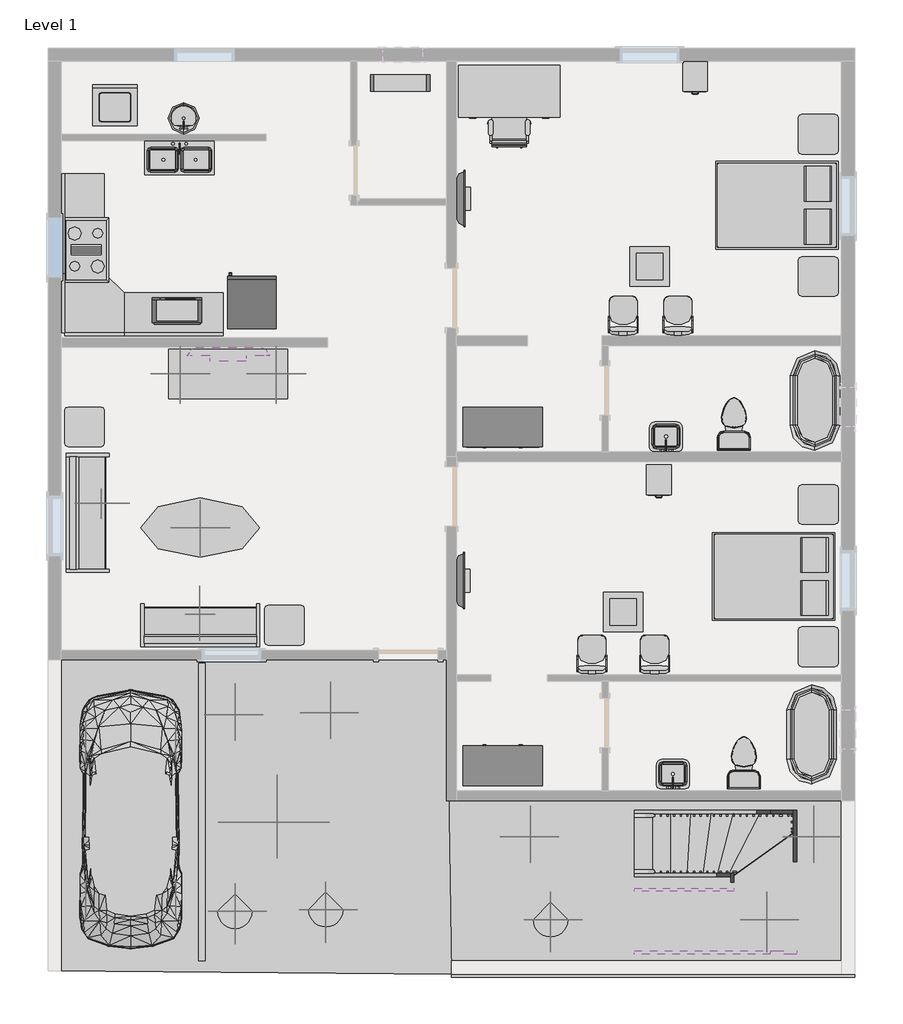
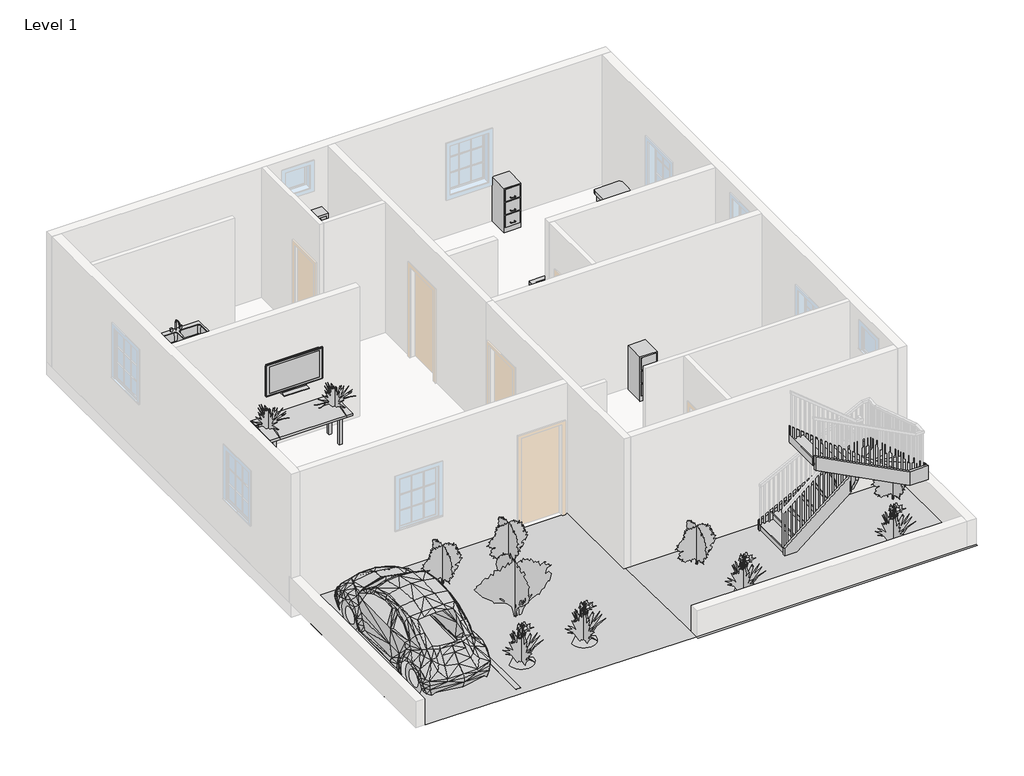
# One storey, part 3 of 3: 29 furniture elements, 12 geographic elements, 10 flow terminals, 10 proxies, 8 members, 1 stair flight.
"""IFC4 building model written with IfcOpenShell, lengths in millimetres."""

from ifc_helpers import new_model, si_unit, frame, origin, place, context, project, spatial, polyline, outline, extrude, triangles, transform, mapped, element, save
from components import proxy_bb1e6e30, proxy_8a8d5ab2, parking_space_9_x_18_90_deg_85bc4432, rpc_beetle_rpc_beetle_3ce7ba48, rpc_female_69e001fa, proxy_a13a33b2, proxy_718fa39f, flow_terminal_2b63360b, flow_terminal_accce45a, flow_terminal_a53be723, flow_terminal_d49f872f, flow_terminal_62a433f7, toilet_domestic_3d_toilet_domestic_3d_f7549cf7, toilet_domestic_3d_toilet_domestic_3d_183bbd19, flow_terminal_b374fae2, furniture_c8abb964, furniture_552c1472, chair_task_arms_chair_task_arms_fa5a08ef, furniture_013ab306, furniture_9fa109b2, furniture_3d1d9cbc, furniture_417d203a, furniture_a4ffab56, furniture_56245f3a, furniture_fdf74506, furniture_b5c51a22, furniture_027a2ad9, furniture_31d08a24, furniture_a5b052b6, furniture_b89246da, rpc_plant_tropical_55f6ff97, rpc_plant_tropical_6475341c, rpc_plant_tropical_agave_1_5_93a2a214, rpc_plant_tropical_jungle_flame_3_9c4808c2, stair_flight_cc2d1c0a

model = new_model("IFC4")

# Units and contexts
model_context = context("Model", 3, world=origin())
ifc_project = project(units=[si_unit("LENGTHUNIT", "METRE", prefix="MILLI")], contexts=[model_context])

# Site, building, storey
site = spatial("IfcSite", under=ifc_project)
building = spatial("IfcBuilding", under=site)
storey = spatial("IfcBuildingStorey", under=building, Name="Level 1", Elevation=0.0)

# Proxies
placement = place(None, origin())
element("IfcBuildingElementProxy", 1, Name="Building Element Proxy", at=placement, inside=storey, context=model_context, shape_type="Tessellation", body=[
    triangles([(7242.7375626, -2797.2193771, 0.0), (7242.7375626, -5515.0191833, 0.0), (1045.1378048, -5515.0191833, 0.0), (968.9378048, -2797.2193771, 0.0)], [[4, 3, 1], [2, 1, 3]], closed=False),
])
element("IfcBuildingElementProxy", 2, Name="Building Element Proxy", at=placement, inside=storey, context=model_context, shape_type="Tessellation", body=[
    triangles([(-5152.4622437, -638.219256, 0.0), (-5152.4622437, -5413.4195709, 0.0), (968.9378048, -638.219256, 0.0), (1045.1378048, -5464.2193771, 0.0)], [[1, 2, 3], [4, 3, 2]], closed=False),
])
proxy_shape = proxy_bb1e6e30(model_context)
element("IfcBuildingElementProxy", 3, Name="Cook Top-4 Unit : 36\" x 20\"", ObjectType="Cook Top-4 Unit : 36\" x 20\"", at=placement, inside=storey, context=model_context, shape_type="MappedRepresentation", body=[
    mapped(proxy_shape, transform((-4568.2621755, 5660.9807133, 0.0), x_axis=(0.0, 1.0000000000000002, 0.0), y_axis=(-1.0000000000000002, 0.0, 0.0), z_axis=(0.0, 0.0, 1.0))),
])
proxy_2_shape = proxy_8a8d5ab2(model_context)
element("IfcBuildingElementProxy", 4, Name="Microwave : 30\" x 16\" x 18\"", ObjectType="Microwave : 30\" x 16\" x 18\"", at=placement, inside=storey, context=model_context, shape_type="MappedRepresentation", body=[
    mapped(proxy_2_shape, transform((-2670.9692982, 4368.1002075, 0.0), x_axis=(-1.0000000000000004, 0.0, 0.0), y_axis=(0.0, -1.0000000000000004, 0.0), z_axis=(0.0, 0.0, 1.0))),
])
parking_space_9_x_18_90_deg_shape = parking_space_9_x_18_90_deg_85bc4432(model_context)
element("IfcBuildingElementProxy", 5, Name="Parking Space : 9' x 18' - 90 deg", ObjectType="Parking Space : 9' x 18' - 90 deg", at=placement, inside=storey, context=model_context, shape_type="MappedRepresentation", body=[
    mapped(parking_space_9_x_18_90_deg_shape, transform((-2790.2621755, -5261.0192867, 0.0), x_axis=(-0.9999999999999997, 0.0, 0.0), y_axis=(0.0, -0.9999999999999997, 0.0), z_axis=(0.0, 0.0, 1.0))),
])
rpc_beetle_rpc_beetle_shape = rpc_beetle_rpc_beetle_3ce7ba48(model_context)
element("IfcBuildingElementProxy", 6, Name="RPC Beetle : RPC Beetle", ObjectType="RPC Beetle : RPC Beetle", at=placement, inside=storey, context=model_context, shape_type="MappedRepresentation", body=[
    mapped(rpc_beetle_rpc_beetle_shape, transform((-3882.4621755, -4321.2192867, 0.0), x_axis=(1.0, 0.0, 0.0), y_axis=(0.0, 1.0, 0.0), z_axis=(0.0, 0.0, 1.0))),
])
rpc_female_shape = rpc_female_69e001fa(model_context)
element("IfcBuildingElementProxy", 7, Name="RPC Female", ObjectType="RPC Female", at=placement, inside=storey, context=model_context, shape_type="MappedRepresentation", body=[
    mapped(rpc_female_shape, transform((-2815.6621755, 225.3807133, 0.0), x_axis=(-1.0000000000000004, 0.0, 0.0), y_axis=(0.0, -1.0000000000000004, 0.0), z_axis=(0.0, 0.0, 1.0))),
])
element("IfcBuildingElementProxy", 8, Name="RPC Female", ObjectType="RPC Female", at=placement, inside=storey, context=model_context, shape_type="MappedRepresentation", body=[
    mapped(rpc_female_shape, transform((-4174.5621755, 1763.4268083, 0.0), x_axis=(0.0, 1.0000000000000007, 0.0), y_axis=(-1.0000000000000007, 0.0, 0.0), z_axis=(0.0, 0.0, 1.0))),
])
proxy_3_shape = proxy_a13a33b2(model_context)
element("IfcBuildingElementProxy", 9, Name="Refrigerator : 30\" x 32\" RH", ObjectType="Refrigerator : 30\" x 32\" RH", at=placement, inside=storey, context=model_context, shape_type="MappedRepresentation", body=[
    mapped(proxy_3_shape, transform((-2020.3246755, 4840.6317418, 0.0), x_axis=(-1.0000000000000004, 0.0, 0.0), y_axis=(0.0, -1.0000000000000004, 0.0), z_axis=(0.0, 0.0, 1.0))),
])
proxy_4_shape = proxy_718fa39f(model_context)
element("IfcBuildingElementProxy", 10, Name="Washer : 27\" x 25\" x 35\"", ObjectType="Washer : 27\" x 25\" x 35\"", at=placement, inside=storey, context=model_context, shape_type="MappedRepresentation", body=[
    mapped(proxy_4_shape, transform((-4544.179644, 7604.3311485, 0.0), x_axis=(1.0, 0.0, 0.0), y_axis=(0.0, 1.0, 0.0), z_axis=(0.0, 0.0, 1.0))),
])

# Flow terminals
flow_terminal_shape = flow_terminal_2b63360b(model_context)
element("IfcFlowTerminal", 11, ObjectType="Floor Drain - Rectangular : 5\"x5\" Strainer - 2\" Drain", at=placement, inside=storey, context=model_context, shape_type="MappedRepresentation", body=[
    mapped(flow_terminal_shape, transform((5947.3378245, -1349.4192867, 0.0), x_axis=(1.0, 0.0, 0.0), y_axis=(0.0, 1.0, 0.0), z_axis=(0.0, 0.0, 1.0))),
])
flow_terminal_2_shape = flow_terminal_accce45a(model_context)
element("IfcFlowTerminal", 12, ObjectType="Floor Drain - Round : 5\" Strainer - 2\" Drain", at=placement, inside=storey, context=model_context, shape_type="MappedRepresentation", body=[
    mapped(flow_terminal_2_shape, transform((-3577.6621755, 7743.7807133, 0.0), x_axis=(1.0, 0.0, 0.0), y_axis=(0.0, 1.0, 0.0), z_axis=(0.0, 0.0, 1.0))),
])
flow_terminal_3_shape = flow_terminal_a53be723(model_context)
element("IfcFlowTerminal", 13, ObjectType="Sink Kitchen-Double : 42\" x 21\"", at=placement, inside=storey, context=model_context, shape_type="MappedRepresentation", body=[
    mapped(flow_terminal_3_shape, transform((-3148.8514161, 7081.0353122, 0.0), x_axis=(1.0, 0.0, 0.0), y_axis=(0.0, 1.0, 0.0), z_axis=(0.0, 0.0, 1.0))),
])
flow_terminal_4_shape = flow_terminal_d49f872f(model_context)
element("IfcFlowTerminal", 14, ObjectType="Sink Vanity-Round : 19\" x 19\"", at=placement, inside=storey, context=model_context, shape_type="MappedRepresentation", body=[
    mapped(flow_terminal_4_shape, transform((-2973.010435, 7767.9535765, 0.0), x_axis=(-1.0000000000000004, 0.0, 0.0), y_axis=(0.0, -1.0000000000000004, 0.0), z_axis=(0.0, 0.0, 1.0))),
])
flow_terminal_5_shape = flow_terminal_62a433f7(model_context)
element("IfcFlowTerminal", 15, ObjectType="Sink Vanity-Square : 20\" x 18\"", at=placement, inside=storey, context=model_context, shape_type="MappedRepresentation", body=[
    mapped(flow_terminal_5_shape, transform((4464.427065, -2439.2738856, 0.0), x_axis=(-0.9999999999999998, 0.0, 0.0), y_axis=(0.0, -0.9999999999999998, 0.0), z_axis=(0.0, 0.0, 1.0))),
])
element("IfcFlowTerminal", 16, ObjectType="Sink Vanity-Square : 20\" x 18\"", at=placement, inside=storey, context=model_context, shape_type="MappedRepresentation", body=[
    mapped(flow_terminal_5_shape, transform((4359.2912059, 2742.3261144, 0.0), x_axis=(-1.0, 0.0, 0.0), y_axis=(0.0, -1.0, 0.0), z_axis=(0.0, 0.0, 1.0))),
])
toilet_domestic_3d_toilet_domestic_3d_shape = toilet_domestic_3d_toilet_domestic_3d_f7549cf7(model_context)
toilet_domestic_3d_toilet_domestic_3d_2_shape = toilet_domestic_3d_toilet_domestic_3d_183bbd19(model_context)
element("IfcFlowTerminal", 17, ObjectType="Toilet-Domestic-3D : Toilet-Domestic-3D", at=placement, inside=storey, context=model_context, shape_type="MappedRepresentation", body=[
    mapped(toilet_domestic_3d_toilet_domestic_3d_shape, transform((5540.9378245, -2124.7232593, 0.0), x_axis=(-1.0000000000000004, 0.0, 0.0), y_axis=(0.0, -1.0000000000000004, 0.0), z_axis=(0.0, 0.0, 1.0))),
    mapped(toilet_domestic_3d_toilet_domestic_3d_2_shape, transform((5540.9378245, -2124.7232593, 0.0), x_axis=(-1.0000000000000004, 0.0, 0.0), y_axis=(0.0, -1.0000000000000004, 0.0), z_axis=(0.0, 0.0, 1.0))),
])
element("IfcFlowTerminal", 18, ObjectType="Toilet-Domestic-3D : Toilet-Domestic-3D", at=placement, inside=storey, context=model_context, shape_type="MappedRepresentation", body=[
    mapped(toilet_domestic_3d_toilet_domestic_3d_shape, transform((5388.5378245, 3082.2767407, 0.0), x_axis=(-1.0000000000000002, 0.0, 0.0), y_axis=(0.0, -1.0000000000000002, 0.0), z_axis=(0.0, 0.0, 1.0))),
    mapped(toilet_domestic_3d_toilet_domestic_3d_2_shape, transform((5388.5378245, 3082.2767407, 0.0), x_axis=(-1.0000000000000002, 0.0, 0.0), y_axis=(0.0, -1.0000000000000002, 0.0), z_axis=(0.0, 0.0, 1.0))),
])
flow_terminal_6_shape = flow_terminal_b374fae2(model_context)
element("IfcFlowTerminal", 19, ObjectType="Tub-Free Standing-3D : 30\" x 60\"", at=placement, inside=storey, context=model_context, shape_type="MappedRepresentation", body=[
    mapped(flow_terminal_6_shape, transform((6582.3378245, -1781.2192867, 0.0), x_axis=(1.0000000000000007, 0.0, 0.0), y_axis=(0.0, 1.0000000000000007, 0.0), z_axis=(0.0, 0.0, 1.0))),
])
element("IfcFlowTerminal", 20, ObjectType="Tub-Free Standing-3D : 30\" x 60\"", at=placement, inside=storey, context=model_context, shape_type="MappedRepresentation", body=[
    mapped(flow_terminal_6_shape, transform((6633.1378245, 3349.5807133, 0.0), x_axis=(1.0, 0.0, 0.0), y_axis=(0.0, 1.0, 0.0), z_axis=(0.0, 0.0, 1.0))),
])

# Furniture
furniture_shape = furniture_c8abb964(model_context)
element("IfcFurniture", 21, ObjectType="Bed-Box : Double 53\" x 74\"", at=placement, inside=storey, context=model_context, shape_type="MappedRepresentation", body=[
    mapped(furniture_shape, transform((6232.5673326, 983.6331723, 0.0), x_axis=(0.0, -0.9999999999999998, 0.0), y_axis=(0.9999999999999998, 0.0, 0.0), z_axis=(0.0, 0.0, 1.0))),
])
element("IfcFurniture", 22, ObjectType="Bed-Box : Double 53\" x 74\"", at=placement, inside=storey, context=model_context, shape_type="MappedRepresentation", body=[
    mapped(furniture_shape, transform((6283.3673326, 6685.9331723, 0.0), x_axis=(0.0, -1.0, 0.0), y_axis=(1.0, 0.0, 0.0), z_axis=(0.0, 0.0, 1.0))),
])
furniture_2_shape = furniture_552c1472(model_context)
element("IfcFurniture", 23, ObjectType="Cabinet-File 3 Drawer : 15\" x 18\"", at=placement, inside=storey, context=model_context, shape_type="MappedRepresentation", body=[
    mapped(furniture_2_shape, transform((4360.7342715, 2272.5150134, 0.0), x_axis=(1.0, 0.0, 0.0), y_axis=(0.0, 1.0, 0.0), z_axis=(0.0, 0.0, 1.0))),
])
element("IfcFurniture", 24, ObjectType="Cabinet-File 3 Drawer : 15\" x 18\"", at=placement, inside=storey, context=model_context, shape_type="MappedRepresentation", body=[
    mapped(furniture_2_shape, transform((4919.5342715, 8470.1150134, 0.0), x_axis=(1.0, 0.0, 0.0), y_axis=(0.0, 1.0, 0.0), z_axis=(0.0, 0.0, 1.0))),
])
chair_task_arms_chair_task_arms_shape = chair_task_arms_chair_task_arms_fa5a08ef(model_context)
element("IfcFurniture", 25, ObjectType="Chair-Task Arms : Chair-Task Arms", at=placement, inside=storey, context=model_context, shape_type="MappedRepresentation", body=[
    mapped(chair_task_arms_chair_task_arms_shape, transform((1793.1470048, 7496.2348117, 0.0), x_axis=(1.0, 0.0, 0.0), y_axis=(0.0, 1.0, 0.0), z_axis=(0.0, 0.0, 1.0))),
])
furniture_3_shape = furniture_013ab306(model_context)
element("IfcFurniture", 26, ObjectType="Desk : 60\" x 30\"", at=placement, inside=storey, context=model_context, shape_type="MappedRepresentation", body=[
    mapped(furniture_3_shape, transform((1172.1378245, 7718.3807133, 0.0), x_axis=(1.0, 0.0, 0.0), y_axis=(0.0, 1.0, 0.0), z_axis=(0.0, 0.0, 1.0))),
])
furniture_4_shape = furniture_9fa109b2(model_context)
element("IfcFurniture", 27, ObjectType="Dresser : 48\" x 72\" x 24\"", at=placement, inside=storey, context=model_context, shape_type="MappedRepresentation", body=[
    mapped(furniture_4_shape, transform((1563.3445646, -2626.9822408, 0.0), x_axis=(-1.0, 0.0, 0.0), y_axis=(0.0, -1.0, 0.0), z_axis=(0.0, 0.0, 1.0))),
])
element("IfcFurniture", 28, ObjectType="Dresser : 48\" x 72\" x 24\"", at=placement, inside=storey, context=model_context, shape_type="MappedRepresentation", body=[
    mapped(furniture_4_shape, transform((2101.7310843, 3306.3436674, 0.0), x_axis=(1.0, 0.0, 0.0), y_axis=(0.0, 1.0, 0.0), z_axis=(0.0, 0.0, 1.0))),
])
furniture_5_shape = furniture_3d1d9cbc(model_context)
element("IfcFurniture", 29, ObjectType="Seating-Auditorium : 18\" x 24\" x 30\"", at=placement, inside=storey, context=model_context, shape_type="MappedRepresentation", body=[
    mapped(furniture_5_shape, transform((4008.6099556, -751.8946965, 0.0), x_axis=(1.0, 0.0, 0.0), y_axis=(0.0, 1.0, 0.0), z_axis=(0.0, 0.0, 1.0))),
])
element("IfcFurniture", 30, ObjectType="Seating-Auditorium : 18\" x 24\" x 30\"", at=placement, inside=storey, context=model_context, shape_type="MappedRepresentation", body=[
    mapped(furniture_5_shape, transform((3043.4099556, -751.8946965, 0.0), x_axis=(1.0, 0.0, 0.0), y_axis=(0.0, 1.0, 0.0), z_axis=(0.0, 0.0, 1.0))),
])
element("IfcFurniture", 31, ObjectType="Seating-Auditorium : 18\" x 24\" x 30\"", at=placement, inside=storey, context=model_context, shape_type="MappedRepresentation", body=[
    mapped(furniture_5_shape, transform((4364.2099556, 4455.1053035, 0.0), x_axis=(1.0, 0.0, 0.0), y_axis=(0.0, 1.0, 0.0), z_axis=(0.0, 0.0, 1.0))),
])
element("IfcFurniture", 32, ObjectType="Seating-Auditorium : 18\" x 24\" x 30\"", at=placement, inside=storey, context=model_context, shape_type="MappedRepresentation", body=[
    mapped(furniture_5_shape, transform((3526.0099556, 4455.1053035, 0.0), x_axis=(1.0, 0.0, 0.0), y_axis=(0.0, 1.0, 0.0), z_axis=(0.0, 0.0, 1.0))),
])
furniture_6_shape = furniture_417d203a(model_context)
element("IfcFurniture", 33, ObjectType="Shelving : 36\" x 10\" x 72\"", at=placement, inside=storey, context=model_context, shape_type="MappedRepresentation", body=[
    mapped(furniture_6_shape, transform((257.7378245, 8531.1807133, 0.0), x_axis=(1.0, 0.0, 0.0), y_axis=(0.0, 1.0, 0.0), z_axis=(0.0, 0.0, 1.0))),
])
furniture_7_shape = furniture_a4ffab56(model_context)
element("IfcFurniture", 34, ObjectType="Sofa : 72\"", at=placement, inside=storey, context=model_context, shape_type="MappedRepresentation", body=[
    mapped(furniture_7_shape, transform((-4396.7080772, 1552.0102215, 0.0), x_axis=(0.0, 1.0000000000000009, 0.0), y_axis=(-1.0000000000000009, 0.0, 0.0), z_axis=(0.0, 0.0, 1.0))),
])
element("IfcFurniture", 35, ObjectType="Sofa : 72\"", at=placement, inside=storey, context=model_context, shape_type="MappedRepresentation", body=[
    mapped(furniture_7_shape, transform((-2745.2916837, 41.3348117, 0.0), x_axis=(-1.0000000000000004, 0.0, 0.0), y_axis=(0.0, -1.0000000000000004, 0.0), z_axis=(0.0, 0.0, 1.0))),
])
furniture_8_shape = furniture_56245f3a(model_context)
element("IfcFurniture", 36, ObjectType="TV - Flat Screen : 32\"", at=placement, inside=storey, context=model_context, shape_type="MappedRepresentation", body=[
    mapped(furniture_8_shape, transform((1179.7082118, 584.9252275, 1041.4), x_axis=(0.0, 1.0, 0.0), y_axis=(-1.0, 0.0, 0.0), z_axis=(0.0, 0.0, 1.0))),
])
element("IfcFurniture", 37, ObjectType="TV - Flat Screen : 32\"", at=placement, inside=storey, context=model_context, shape_type="MappedRepresentation", body=[
    mapped(furniture_8_shape, transform((1184.7140608, 6452.3252275, 914.4), x_axis=(0.0, 1.0000000000000002, 0.0), y_axis=(-1.0000000000000002, 0.0, 0.0), z_axis=(0.0, 0.0, 1.0))),
])
furniture_9_shape = furniture_fdf74506(model_context)
element("IfcFurniture", 38, ObjectType="TV - Flat Screen : 50\"", at=placement, inside=storey, context=model_context, shape_type="MappedRepresentation", body=[
    mapped(furniture_9_shape, transform((-2379.9176614, 4104.4863058, 1219.2), x_axis=(1.0, 0.0, 0.0), y_axis=(0.0, 1.0, 0.0), z_axis=(0.0, 0.0, 1.0))),
])
furniture_10_shape = furniture_b5c51a22(model_context)
element("IfcFurniture", 39, ObjectType="Table-Coffee : 24\" x 24\" x 24\"", at=placement, inside=storey, context=model_context, shape_type="MappedRepresentation", body=[
    mapped(furniture_10_shape, transform((3668.4720578, 3.1696355, 0.0), x_axis=(1.0, 0.0, 0.0), y_axis=(0.0, 1.0, 0.0), z_axis=(0.0, 0.0, 1.0))),
])
element("IfcFurniture", 40, ObjectType="Table-Coffee : 24\" x 24\" x 24\"", at=placement, inside=storey, context=model_context, shape_type="MappedRepresentation", body=[
    mapped(furniture_10_shape, transform((4074.8720578, 5311.7696355, 0.0), x_axis=(1.0, 0.0, 0.0), y_axis=(0.0, 1.0, 0.0), z_axis=(0.0, 0.0, 1.0))),
])
furniture_11_shape = furniture_027a2ad9(model_context)
element("IfcFurniture", 41, ObjectType="Table-Ellipse : 72\" x 36\"", at=placement, inside=storey, context=model_context, shape_type="MappedRepresentation", body=[
    mapped(furniture_11_shape, transform((-2815.6621755, 1393.7807133, 0.0), x_axis=(-1.0000000000000002, 0.0, 0.0), y_axis=(0.0, -1.0000000000000002, 0.0), z_axis=(0.0, 0.0, 1.0))),
])
furniture_12_shape = furniture_31d08a24(model_context)
element("IfcFurniture", 42, ObjectType="Table-End : 24\" x 24\"", at=placement, inside=storey, context=model_context, shape_type="MappedRepresentation", body=[
    mapped(furniture_12_shape, transform((-1828.7958058, -257.2192867, 0.0), x_axis=(1.0, 0.0, 0.0), y_axis=(0.0, 1.0, 0.0), z_axis=(0.0, 0.0, 1.0))),
])
element("IfcFurniture", 43, ObjectType="Table-End : 24\" x 24\"", at=placement, inside=storey, context=model_context, shape_type="MappedRepresentation", body=[
    mapped(furniture_12_shape, transform((-4902.1958058, 2790.7807133, 0.0), x_axis=(1.0, 0.0, 0.0), y_axis=(0.0, 1.0, 0.0), z_axis=(0.0, 0.0, 1.0))),
])
element("IfcFurniture", 44, ObjectType="Table-End : 24\" x 24\"", at=placement, inside=storey, context=model_context, shape_type="MappedRepresentation", body=[
    mapped(furniture_12_shape, transform((6375.4041942, 1596.9807133, 0.0), x_axis=(1.0, 0.0, 0.0), y_axis=(0.0, 1.0, 0.0), z_axis=(0.0, 0.0, 1.0))),
])
element("IfcFurniture", 45, ObjectType="Table-End : 24\" x 24\"", at=placement, inside=storey, context=model_context, shape_type="MappedRepresentation", body=[
    mapped(furniture_12_shape, transform((6375.4041942, -587.4192867, 0.0), x_axis=(1.0, 0.0, 0.0), y_axis=(0.0, 1.0, 0.0), z_axis=(0.0, 0.0, 1.0))),
])
element("IfcFurniture", 46, ObjectType="Table-End : 24\" x 24\"", at=placement, inside=storey, context=model_context, shape_type="MappedRepresentation", body=[
    mapped(furniture_12_shape, transform((6375.4041942, 5102.1807133, 0.0), x_axis=(1.0, 0.0, 0.0), y_axis=(0.0, 1.0, 0.0), z_axis=(0.0, 0.0, 1.0))),
])
element("IfcFurniture", 47, ObjectType="Table-End : 24\" x 24\"", at=placement, inside=storey, context=model_context, shape_type="MappedRepresentation", body=[
    mapped(furniture_12_shape, transform((6375.4041942, 7286.5807133, 0.0), x_axis=(1.0, 0.0, 0.0), y_axis=(0.0, 1.0, 0.0), z_axis=(0.0, 0.0, 1.0))),
])
furniture_13_shape = furniture_a5b052b6(model_context)
element("IfcFurniture", 48, ObjectType="Table-Rectangular : 72\" x 30\"", at=placement, inside=storey, context=model_context, shape_type="MappedRepresentation", body=[
    mapped(furniture_13_shape, transform((-2383.8621755, 3755.9807133, 0.0), x_axis=(1.0, 0.0, 0.0), y_axis=(0.0, 1.0, 0.0), z_axis=(0.0, 0.0, 1.0))),
])
furniture_14_shape = furniture_b89246da(model_context)
element("IfcFurniture", 49, ObjectType="Work Station Cubicle : 96\" x 96\"", at=placement, inside=storey, context=model_context, shape_type="MappedRepresentation", body=[
    mapped(furniture_14_shape, transform((-5444.2851832, 4471.9124655, 0.0), x_axis=(0.0, 1.0000000000000002, 0.0), y_axis=(-1.0000000000000002, 0.0, 0.0), z_axis=(0.0, 0.0, 1.0))),
])

# Geographic elements
rpc_plant_tropical_shape = rpc_plant_tropical_55f6ff97(model_context)
element("IfcGeographicElement", 50, ObjectType="RPC Plant - Tropical", at=placement, inside=storey, context=model_context, shape_type="MappedRepresentation", body=[
    mapped(rpc_plant_tropical_shape, transform((-2282.2621755, -4499.0192867, 0.0), x_axis=(1.0, 0.0, 0.0), y_axis=(0.0, 1.0, 0.0), z_axis=(0.0, 0.0, 1.0))),
])
element("IfcGeographicElement", 51, ObjectType="RPC Plant - Tropical", at=placement, inside=storey, context=model_context, shape_type="MappedRepresentation", body=[
    mapped(rpc_plant_tropical_shape, transform((5896.5378245, -4626.0192867, 0.0), x_axis=(1.0, 0.0, 0.0), y_axis=(0.0, 1.0, 0.0), z_axis=(0.0, 0.0, 1.0))),
])
element("IfcGeographicElement", 52, ObjectType="RPC Plant - Tropical", at=placement, inside=storey, context=model_context, shape_type="MappedRepresentation", body=[
    mapped(rpc_plant_tropical_shape, transform((2569.1378245, -4626.0192867, 0.0), x_axis=(1.0, 0.0, 0.0), y_axis=(0.0, 1.0, 0.0), z_axis=(0.0, 0.0, 1.0))),
])
element("IfcGeographicElement", 53, ObjectType="RPC Plant - Tropical", at=placement, inside=storey, context=model_context, shape_type="MappedRepresentation", body=[
    mapped(rpc_plant_tropical_shape, transform((-885.2621755, -4473.6192867, 0.0), x_axis=(1.0, 0.0, 0.0), y_axis=(0.0, 1.0, 0.0), z_axis=(0.0, 0.0, 1.0))),
])
rpc_plant_tropical_2_shape = rpc_plant_tropical_6475341c(model_context)
element("IfcGeographicElement", 54, ObjectType="RPC Plant - Tropical", at=placement, inside=storey, context=model_context, shape_type="MappedRepresentation", body=[
    mapped(rpc_plant_tropical_2_shape, transform((-1571.0621755, -3127.4192867, 0.0), x_axis=(1.0, 0.0, 0.0), y_axis=(0.0, 1.0, 0.0), z_axis=(0.0, 0.0, 1.0))),
])
rpc_plant_tropical_agave_1_5_shape = rpc_plant_tropical_agave_1_5_93a2a214(model_context)
element("IfcGeographicElement", 55, ObjectType="RPC Plant - Tropical : Agave - 1.5'", at=placement, inside=storey, context=model_context, shape_type="MappedRepresentation", body=[
    mapped(rpc_plant_tropical_agave_1_5_shape, transform((-2815.6621755, 1393.7807133, 762.0), x_axis=(1.0, 0.0, 0.0), y_axis=(0.0, 1.0, 0.0), z_axis=(0.0, 0.0, 1.0))),
])
element("IfcGeographicElement", 56, ObjectType="RPC Plant - Tropical : Agave - 1.5'", at=placement, inside=storey, context=model_context, shape_type="MappedRepresentation", body=[
    mapped(rpc_plant_tropical_agave_1_5_shape, transform((-3120.4621755, 3755.9807133, 762.0), x_axis=(1.0, 0.0, 0.0), y_axis=(0.0, 1.0, 0.0), z_axis=(0.0, 0.0, 1.0))),
])
element("IfcGeographicElement", 57, ObjectType="RPC Plant - Tropical : Agave - 1.5'", at=placement, inside=storey, context=model_context, shape_type="MappedRepresentation", body=[
    mapped(rpc_plant_tropical_agave_1_5_shape, transform((-1647.2621755, 3755.9807133, 762.0), x_axis=(1.0, 0.0, 0.0), y_axis=(0.0, 1.0, 0.0), z_axis=(0.0, 0.0, 1.0))),
])
rpc_plant_tropical_jungle_flame_3_shape = rpc_plant_tropical_jungle_flame_3_9c4808c2(model_context)
element("IfcGeographicElement", 58, ObjectType="RPC Plant - Tropical : Jungle Flame - 3'", at=placement, inside=storey, context=model_context, shape_type="MappedRepresentation", body=[
    mapped(rpc_plant_tropical_jungle_flame_3_shape, transform((-2282.2621755, -1476.4192867, 0.0), x_axis=(1.0, 0.0, 0.0), y_axis=(0.0, 1.0, 0.0), z_axis=(0.0, 0.0, 1.0))),
])
element("IfcGeographicElement", 59, ObjectType="RPC Plant - Tropical : Jungle Flame - 3'", at=placement, inside=storey, context=model_context, shape_type="MappedRepresentation", body=[
    mapped(rpc_plant_tropical_jungle_flame_3_shape, transform((2264.3378245, -3356.0192867, 0.0), x_axis=(1.0, 0.0, 0.0), y_axis=(0.0, 1.0, 0.0), z_axis=(0.0, 0.0, 1.0))),
])
element("IfcGeographicElement", 60, ObjectType="RPC Plant - Tropical : Jungle Flame - 3'", at=placement, inside=storey, context=model_context, shape_type="MappedRepresentation", body=[
    mapped(rpc_plant_tropical_jungle_flame_3_shape, transform((6614.0878245, -3356.0192867, 0.0), x_axis=(1.0, 0.0, 0.0), y_axis=(0.0, 1.0, 0.0), z_axis=(0.0, 0.0, 1.0))),
])
element("IfcGeographicElement", 61, ObjectType="RPC Plant - Tropical : Jungle Flame - 3'", at=placement, inside=storey, context=model_context, shape_type="MappedRepresentation", body=[
    mapped(rpc_plant_tropical_jungle_flame_3_shape, transform((-809.0621755, -1451.0192867, 0.0), x_axis=(1.0, 0.0, 0.0), y_axis=(0.0, 1.0, 0.0), z_axis=(0.0, 0.0, 1.0))),
])

# Members
element("IfcMember", 62, ObjectType="Stringer - 2\" Width", at=placement, inside=storey, context=model_context, shape_type="SweptSolid", body=[
    extrude(outline(polyline([(229.639954, 3860.8061326), (0.0, 3860.8061326), (0.0, 4080.5684502), (962.500629, 5948.2233243), (1305.3956453, 5948.2233243), (229.639954, 3860.8061326)])), frame((0.0, -3000.4192867, 0.0), z_axis=(0.0, 1.0, 0.0), x_axis=(0.0, 0.0, 1.0)), (0.0, 0.0, 1.0), 50.8),
])
element("IfcMember", 63, ObjectType="Stringer - 2\" Width", at=placement, inside=storey, context=model_context, shape_type="SweptSolid", body=[
    extrude(outline(polyline([(5948.2233243, -3000.4192867), (5948.2233243, -2949.6192867), (6302.9378245, -2949.6192867), (6302.9378245, -3000.4192867), (5948.2233243, -3000.4192867)])), frame((0.0, 0.0, 962.500629), z_axis=(0.0, 0.0, 1.0), x_axis=(1.0, 0.0, 0.0)), (0.0, 0.0, 1.0), 342.8950162),
])
element("IfcMember", 64, ObjectType="Stringer - 2\" Width", at=placement, inside=storey, context=model_context, shape_type="SweptSolid", body=[
    extrude(outline(polyline([(-2949.6192867, 1289.0952212), (-2949.6192867, 1000.5956453), (-3119.1417696, 1000.5956453), (-5108.6192867, 1638.9682298), (-5108.6192867, 1969.9972697), (-5071.6391694, 1969.9972697), (-2949.6192867, 1289.0952212)])), frame((6302.9378245, 0.0, 0.0), z_axis=(1.0, 0.0, 0.0), x_axis=(0.0, 1.0, 0.0)), (0.0, 0.0, 1.0), 50.8),
])
element("IfcMember", 65, ObjectType="Stringer - 2\" Width", at=placement, inside=storey, context=model_context, shape_type="SweptSolid", body=[
    extrude(outline(polyline([(6353.7378245, -5108.6192867), (6353.7378245, -5159.4192867), (5948.2233243, -5159.4192867), (5948.2233243, -5108.6192867), (6353.7378245, -5108.6192867)])), frame((0.0, 0.0, 1649.8904473), z_axis=(0.0, 0.0, 1.0), x_axis=(1.0, 0.0, 0.0)), (0.0, 0.0, 1.0), 320.1068224),
])
element("IfcMember", 66, ObjectType="Stringer - 2\" Width", at=placement, inside=storey, context=model_context, shape_type="SweptSolid", body=[
    extrude(outline(polyline([(1649.8904473, 5948.2233243), (1969.9972697, 5948.2233243), (3045.7529609, 3860.8061326), (2725.6461385, 3860.8061326), (1649.8904473, 5948.2233243)])), frame((0.0, -5159.4192867, 0.0), z_axis=(0.0, 1.0, 0.0), x_axis=(0.0, 0.0, 1.0)), (0.0, 0.0, 1.0), 50.8),
])
element("IfcMember", 67, ObjectType="Stringer - 2\" Width", at=placement, inside=storey, context=model_context, shape_type="SweptSolid", body=[
    extrude(outline(polyline([(176.1764461, 3860.8061326), (0.0, 3860.8061326), (0.0, 4127.0677771), (987.1410923, 5337.7378245), (1380.418648, 5337.7378245), (176.1764461, 3860.8061326)])), frame((0.0, -3965.6192867, 0.0), z_axis=(0.0, 1.0, 0.0), x_axis=(0.0, 0.0, 1.0)), (0.0, 0.0, 1.0), 50.8),
])
element("IfcMember", 68, ObjectType="Stringer - 2\" Width", at=placement, inside=storey, context=model_context, shape_type="SweptSolid", body=[
    extrude(outline(polyline([(-3914.8192867, 1573.2682978), (-3914.8192867, 1028.5617647), (-3949.061504, 1028.5617647), (-4143.4192867, 1360.465107), (-4143.4192867, 1926.1409689), (-4121.4564041, 1926.1409689), (-3914.8192867, 1573.2682978)])), frame((5337.7378245, 0.0, 0.0), z_axis=(1.0, 0.0, 0.0), x_axis=(0.0, 1.0, 0.0)), (0.0, 0.0, 1.0), 50.8),
])
element("IfcMember", 69, ObjectType="Stringer - 2\" Width", at=placement, inside=storey, context=model_context, shape_type="SweptSolid", body=[
    extrude(outline(polyline([(1532.8634131, 5388.5378245), (1926.1409689, 5388.5378245), (3171.8038432, 3860.8061326), (2778.5262875, 3860.8061326), (1532.8634131, 5388.5378245)])), frame((0.0, -4194.2192867, 0.0), z_axis=(0.0, 1.0, 0.0), x_axis=(0.0, 0.0, 1.0)), (0.0, 0.0, 1.0), 50.8),
])

# Stair flight
stair_flight_shape = stair_flight_cc2d1c0a(model_context)
element("IfcStairFlight", 70, ObjectType="2\" Tread 1\" Nosing 1/4\" Riser", at=placement, inside=storey, context=model_context, shape_type="MappedRepresentation", body=[
    mapped(stair_flight_shape, transform((0.0, 0.0, 0.0), x_axis=(1.0, 0.0, 0.0), y_axis=(0.0, 1.0, 0.0), z_axis=(0.0, 0.0, 1.0))),
])

save(model, "model.ifc")

# Revit data of these elements
# Type "Cook Top-4 Unit : 36\" x 20\""
#   Assembly Code = "E1090400"
#   Depth = 2' - 0"
#   Width = 3' - 0"
#   Burner Material = Steel, Chrome Plated
#   Cooktop Material = Steel, Polished
#   Default Elevation = 0
# Type "Microwave : 30\" x 16\" x 18\""
#   Assembly Code = "E1090400"
#   Depth = 1' - 4"
#   Height = 1' - 6"
#   Width = 2' - 6"
#   Microwave Material = Laminate, Ivory, Matte
#   Default Elevation = 0
# Type "Parking Space : 9' x 18' - 90 deg"
#   Angle = 90.00°
#   Parking Length = 14' - 0"
#   Parking Width = 9' - 0"
#   pl = 15' - 0"
#   pw = 7' - 0"
# Type "RPC Beetle : RPC Beetle"
#   built-in parameter 1005195 = "RPC-16-0U6E-L4EG-ENH1-J3KF-SVEL-0TX4-C0"
#   Height = 0
# Type "RPC Female"
#   built-in parameter 1005195 = "RPC-8-FXA2-QQQ0-UGV2-6"
#   Height = 0
# Type "Refrigerator : 30\" x 32\" RH"
#   Label = "REF."
#   Assembly Code = "E1090400"
#   Depth = 2' - 7 3/4"
#   Handle = 2' - 3"
#   Height = 5' - 10"
#   Rear Clearance = 0' - 2"
#   Top Door Height = 1' - 8"
#   Width = 2' - 5 3/8"
#   Material = Steel, Paint Finish, Ivory, Glossy
#   Default Elevation = 0
# Type "Washer : 27\" x 25\" x 35\""
#   Label = "W"
#   Assembly Code = "E1090400"
#   Depth = 2' - 1"
#   Height = 2' - 11"
#   Width = 2' - 3"
#   Washer Material = Steel, Paint Finish, Ivory, Matte
#   Default Elevation = 0
# Type "Floor Drain - Rectangular : 5\"x5\" Strainer - 2\" Drain"
#   WFU = 2
#   Strainer Height = 0' - 3 1/4"
#   Half Strainer Length = 0' - 2 1/2"
#   Strainer Length = 0' - 5"
#   Radius 2 = 0' - 3.04167"
#   Radius 1 = 0' - 2.02083"
#   Radius 3 = 0' - 2 1/32"
#   Pipe Radius = 1"
#   Pipe Diameter = 2"
#   Height 2 = 0' - 0.725"
#   Height 1 = 0' - 1 13/16"
#   Body Radius = 0' - 4 1/16"
#   Body Height = 0' - 3 5/8"
#   Body Diameter = 0' - 8 1/8"
#   Drain Material = none
#   HWFU = 0
#   Default Elevation = 0
#   CWFU = 0
# Type "Floor Drain - Round : 5\" Strainer - 2\" Drain"
#   WFU = 2
#   Strainer Height = 0' - 3 1/4"
#   Strainer Radius = 0' - 2 1/2"
#   Strainer Diameter = 0' - 5"
#   Radius 6 = 0' - 0 5/8"
#   Radius 5 = 0' - 1 1/4"
#   Radius 4 = 0' - 1 7/8"
#   Radius 2 = 0' - 3.04167"
#   Radius 1 = 0' - 2.02083"
#   Radius 3 = 0' - 2 1/32"
#   Pipe Radius = 1"
#   Pipe Diameter = 2"
#   Height 2 = 0' - 0.725"
#   Height 1 = 0' - 1 13/16"
#   Body Radius = 0' - 4 1/16"
#   Body Height = 0' - 3 5/8"
#   Body Diameter = 0' - 8 1/8"
#   Drain Material = none
#   HWFU = 0
#   Default Elevation = 0
#   CWFU = 0
# Type "Sink Kitchen-Double : 42\" x 21\""
#   Assembly Code = "D2010410"
#   Counter Height = 3' - 0"
#   Depth = 1' - 9"
#   Width = 3' - 6"
#   Faucet Material = Steel, Polished
#   Sink Material = Steel, Polished
#   Default Elevation = 0
# Type "Sink Vanity-Round : 19\" x 19\""
#   Assembly Code = "D2010400"
#   Top Of Counter = 2' - 7"
#   Basin Material = Porcelain, Linen
#   Faucet Material = Steel, Polished
#   Default Elevation = 0
# Type "Sink Vanity-Square : 20\" x 18\""
#   Assembly Code = "D2010400"
#   Counter Height = 2' - 7"
#   Depth = 1' - 6"
#   Width = 1' - 8"
#   Basin Material = Porcelain, Linen
#   Faucet Material = Steel, Polished
#   Default Elevation = 0
# Type "Toilet-Domestic-3D : Toilet-Domestic-3D"
#   Assembly Code = "D2010110"
#   Toilet - Bowl/Basin Material = Porcelain, Linen
#   Toilet - Seat Material = Laminate, Linen, Matte
#   Default Elevation = 0
# Type "Tub-Free Standing-3D : 30\" x 60\""
#   Assembly Code = "D2010110"
#   Height = 1' - 6"
#   Length = 5' - 0"
#   Width = 2' - 6"
#   Tub Material = Porcelain, Ivory
#   Default Elevation = 0
# Type "Bed-Box : Double 53\" x 74\""
#   Assembly Code = "E2020200"
#   Length = 6' - 2"
#   Width = 4' - 5"
#   Frame Material = Birch
#   Mattress Material = Linen, White
#   Default Elevation = 0
# Type "Cabinet-File 3 Drawer : 15\" x 18\""
#   Assembly Code = "E2020200"
#   Depth = 1' - 6"
#   Height = 3' - 5"
#   Width = 1' - 3"
#   Cabinet Material = Steel, Paint Finish, Ivory, Glossy
#   Handle Material = Steel, Chrome Plated
#   Default Elevation = 0
# Type "Chair-Task Arms : Chair-Task Arms"
#   Assembly Code = "E2020200"
#   Base Material = Plastic, Opaque Black
#   Caster Material = Plastic, Opaque Black
#   Seat/Back Material = Textile - Slate Blue
#   Default Elevation = 0
# Type "Desk : 60\" x 30\""
#   Assembly Code = "E2020200"
#   Depth = 2' - 6"
#   Height = 2' - 6"
#   Leg Height = 0' - 6"
#   Width = 5' - 0"
#   Body Material = Laminate, Ivory, Matte
#   Handle/Leg Material = Steel, Chrome Plated
#   Top Material = Cherry
#   Default Elevation = 0
# Type "Dresser : 48\" x 72\" x 24\""
#   Assembly Code = "E2020200"
#   Depth = 2' - 0"
#   Height = 6' - 0"
#   Width = 4' - 0"
#   Dresser Material = Laminate - Ivory, Glossy
#   Drawer Material = Laminate, Ivory, Matte
#   Knob Material = Cherry
#   Default Elevation = 0
# Type "Seating-Auditorium : 18\" x 24\" x 30\""
#   Assembly Code = "E2020200"
#   Seat Material = Linen, Beige
#   Frame Material = Steel, Paint Finish, Dark Gray, Matte
#   Default Elevation = 0
# Type "Shelving : 36\" x 10\" x 72\""
#   Assembly Code = "E2020200"
#   Depth = 0' - 10"
#   Height = 6' - 0"
#   Width = 3' - 0"
#   Shelving Unit Material = Birch
#   Default Elevation = 0
# Type "Sofa : 72\""
#   Assembly Code = "E2020200"
#   Width = 6' - 0"
#   Seat Material = Leather - Black
#   Frame Material = Carpet (2)
#   Default Elevation = 0
# Type "TV - Flat Screen : 32\""
#   SinAng = 0' - 0.0193"
#   L = 2' - 3.79372"
#   H = 1' - 3.6354"
#   Thickness = 0' - 4.33071"
#   Diagonal = 2' - 7.88976"
#   CosAng = 0' - 0.03431"
#   Stand [instance default] = yes
#   Default Elevation = 0
# Type "TV - Flat Screen : 50\""
#   SinAng = 0' - 0.0193"
#   L = 3' - 7.57782"
#   H = 2' - 0.51477"
#   Thickness = 0' - 4.33071"
#   Diagonal = 4' - 2"
#   CosAng = 0' - 0.03431"
#   Stand [instance default] = yes
#   Default Elevation = 0
# Type "Table-Coffee : 24\" x 24\" x 24\""
#   Assembly Code = "E2020200"
#   Height = 2' - 0"
#   Length = 2' - 0"
#   Width = 2' - 0"
#   Top Material = none
#   Frame Material = none
#   Default Elevation = 0
# Type "Table-Ellipse : 72\" x 36\""
#   Assembly Code = "E2020200"
#   Half Width = 1' - 6"
#   Half Length = 3' - 0"
#   Height = 2' - 6"
#   Length = 6' - 0"
#   Width = 3' - 0"
#   Base Material = Birch
#   Top Material = Gypsum Wall Board
#   Default Elevation = 0
# Type "Table-End : 24\" x 24\""
#   Assembly Code = "E2020200"
#   Height = 2' - 0"
#   Length = 2' - 0"
#   Width = 2' - 0"
#   Base Material = Birch
#   Top Material = Laminate, Ivory, Matte
#   Default Elevation = 0
# Type "Table-Rectangular : 72\" x 30\""
#   Assembly Code = "E2020200"
#   Height = 2' - 6"
#   Length = 6' - 0"
#   Width = 2' - 6"
#   Base Material = Birch
#   Top Material = Birch
#   Default Elevation = 0
# Type "Work Station Cubicle : 96\" x 96\""
#   Assembly Code = "E2020"
#   Desktop Height = 2' - 6"
#   Desktop1 Width = 2' - 0"
#   Desktop2 Width = 2' - 0"
#   Panel Height = 3' - 6"
#   Panel1 Length = 5' - 0"
#   Panel2 Length = 5' - 0"
#   Cube Panel Material = Textile - Light Gray
#   Work Top Material = Laminate, Ivory, Matte
#   Default Elevation = 0
# Type "RPC Plant - Tropical"
#   built-in parameter 1005198 = "{2, 15},{39, RPC-16-FWM5-GM7X-C67P-4000-ST1L-LVER-AU},{1, 0},{1, 0},{2, 13},{1, 8},{5, Color},{1, 0},{1, 0},{3, 0.8},{3, 0.8},{3, 0.8},{1, 8},{7, BBoxMin},{1, 0},{1, 0},{1, 0},{1, 0},{1, 0},{1, 8},{7, BBoxMax},{1, 0},{1, 0},{1, 0},{1, 0},{1, 0},{2, 11},{9, RPCTypeId},{1, 0},{1, 0},{39, RPC-16-FWM5-GM7X-C67P-4000-ST1L-LVER-AU},{1, 6},{14, RPCPlantHeight},{1, 0},{1, 0},{1, 3},{2, 11},{7, keyword},{1, 0},{1, 0},{35, :RPCs:Shrubs [General]:Geometry:RPC},{2, 11},{8, category},{1, 0},{1, 0},{16, Shrubs [General]},{2, 11},{12, LocalizedUID},{1, 0},{1, 0},{10, Crane Lily},{2, 14},{6, Height},{1, 0},{1, 0},{1, 3},{1, 2},{16, Cast Reflections},{1, 0},{1, 0},{1, 0},{1, 2},{12, Cast Shadows},{1, 0},{1, 0},{1, 1},{1, 2},{9, Lock View},{1, 0},{1, 0},{1, 0},{1, 4},{5, ViewC},{1, 0},{1, 0},{1, 0},{21, assetlibrary_base.fbx},{1, 5},"
#   built-in parameter 1005195 = "RPC-16-FWM5-GM7X-C67P-4000-ST1L-LVER-AU"
#   Assembly Code = "G2050500"
#   Height = 3' - 0"
#   Default Elevation = 0
# Type "RPC Plant - Tropical"
#   built-in parameter 1005198 = "{2, 15},{39, RPC-16-G3GK-N2Q0-PN0G-6000-ST1L-LVER-AU},{1, 0},{1, 0},{2, 13},{1, 8},{5, Color},{1, 0},{1, 0},{3, 0.8},{3, 0.8},{3, 0.8},{1, 8},{7, BBoxMin},{1, 0},{1, 0},{1, 0},{1, 0},{1, 0},{1, 8},{7, BBoxMax},{1, 0},{1, 0},{1, 0},{1, 0},{1, 0},{2, 11},{9, RPCTypeId},{1, 0},{1, 0},{39, RPC-16-G3GK-N2Q0-PN0G-6000-ST1L-LVER-AU},{1, 6},{14, RPCPlantHeight},{1, 0},{1, 0},{3, 4.5},{2, 11},{7, keyword},{1, 0},{1, 0},{35, :RPCs:Shrubs [General]:Geometry:RPC},{2, 11},{8, category},{1, 0},{1, 0},{16, Shrubs [General]},{2, 11},{12, LocalizedUID},{1, 0},{1, 0},{12, Honey Myrtle},{2, 14},{6, Height},{1, 0},{1, 0},{3, 4.5},{1, 2},{16, Cast Reflections},{1, 0},{1, 0},{1, 0},{1, 2},{12, Cast Shadows},{1, 0},{1, 0},{1, 1},{1, 2},{9, Lock View},{1, 0},{1, 0},{1, 0},{1, 4},{5, ViewC},{1, 0},{1, 0},{1, 0},{21, assetlibrary_base.fbx},{1, 5},"
#   built-in parameter 1005195 = "RPC-16-G3GK-N2Q0-PN0G-6000-ST1L-LVER-AU"
#   Assembly Code = "G2050500"
#   Height = 4' - 6"
#   Default Elevation = 0
# Type "RPC Plant - Tropical : Agave - 1.5'"
#   built-in parameter 1005198 = "{2, 15},{39, RPC-16-G1GJ-63FX-7K5P-N000-ST1L-LVER-AU},{1, 0},{1, 0},{2, 13},{1, 8},{5, Color},{1, 0},{1, 0},{3, 0.8},{3, 0.8},{3, 0.8},{1, 8},{7, BBoxMin},{1, 0},{1, 0},{1, 0},{1, 0},{1, 0},{1, 8},{7, BBoxMax},{1, 0},{1, 0},{1, 0},{1, 0},{1, 0},{2, 11},{9, RPCTypeId},{1, 0},{1, 0},{39, RPC-16-G1GJ-63FX-7K5P-N000-ST1L-LVER-AU},{1, 6},{14, RPCPlantHeight},{1, 0},{1, 0},{3, 1.5},{2, 11},{7, keyword},{1, 0},{1, 0},{35, :RPCs:Plants [General]:Geometry:RPC},{2, 11},{8, category},{1, 0},{1, 0},{16, Plants [General]},{2, 11},{12, LocalizedUID},{1, 0},{1, 0},{5, Agave},{2, 14},{6, Height},{1, 0},{1, 0},{3, 1.5},{1, 2},{16, Cast Reflections},{1, 0},{1, 0},{1, 0},{1, 2},{12, Cast Shadows},{1, 0},{1, 0},{1, 1},{1, 2},{9, Lock View},{1, 0},{1, 0},{1, 0},{1, 4},{5, ViewC},{1, 0},{1, 0},{1, 0},{21, assetlibrary_base.fbx},{1, 5},"
#   built-in parameter 1005195 = "RPC-16-G1GJ-63FX-7K5P-N000-ST1L-LVER-AU"
#   Type Comments = "Agave"
#   Assembly Code = "G2050500"
#   Height = 1' - 6"
#   Default Elevation = 0
# Type "RPC Plant - Tropical : Jungle Flame - 3'"
#   built-in parameter 1005198 = "{2, 15},{39, RPC-16-FUVJ-JWG0-MWGK-8000-ST1L-LVER-AU},{1, 0},{1, 0},{2, 13},{1, 8},{5, Color},{1, 0},{1, 0},{3, 0.8},{3, 0.8},{3, 0.8},{1, 8},{7, BBoxMin},{1, 0},{1, 0},{1, 0},{1, 0},{1, 0},{1, 8},{7, BBoxMax},{1, 0},{1, 0},{1, 0},{1, 0},{1, 0},{2, 11},{9, RPCTypeId},{1, 0},{1, 0},{39, RPC-16-FUVJ-JWG0-MWGK-8000-ST1L-LVER-AU},{1, 6},{14, RPCPlantHeight},{1, 0},{1, 0},{1, 3},{2, 11},{7, keyword},{1, 0},{1, 0},{35, :RPCs:Shrubs [General]:Geometry:RPC},{2, 11},{8, category},{1, 0},{1, 0},{16, Shrubs [General]},{2, 11},{12, LocalizedUID},{1, 0},{1, 0},{12, Jungle Flame},{2, 14},{6, Height},{1, 0},{1, 0},{1, 3},{1, 2},{16, Cast Reflections},{1, 0},{1, 0},{1, 0},{1, 2},{12, Cast Shadows},{1, 0},{1, 0},{1, 1},{1, 2},{9, Lock View},{1, 0},{1, 0},{1, 0},{1, 4},{5, ViewC},{1, 0},{1, 0},{1, 0},{21, assetlibrary_base.fbx},{1, 5},"
#   built-in parameter 1005195 = "RPC-16-FUVJ-JWG0-MWGK-8000-ST1L-LVER-AU"
#   Type Comments = "Jungle Flame"
#   Assembly Code = "G2050500"
#   Height = 3' - 0"
#   Default Elevation = 0
# Elements 1, 2 (IfcBuildingElementProxy)
#   Material = none
#   Phase Created = New Construction
# Element 3 (IfcBuildingElementProxy, "Cook Top-4 Unit : 36\" x 20\"")
#   Phase Created = New Construction
#   Materials on its faces: "Steel, Chrome Plated", "Steel, Polished"
# Element 4 (IfcBuildingElementProxy, "Microwave : 30\" x 16\" x 18\"")
#   Phase Created = New Construction
#   Materials on its faces: "Laminate, Ivory, Matte", "Glass"
# Element 5 (IfcBuildingElementProxy, "Parking Space : 9' x 18' - 90 deg")
#   Phase Created = New Construction
#   Materials on its faces: "Parking Stripe"
# Element 6 (IfcBuildingElementProxy, "RPC Beetle : RPC Beetle")
#   Phase Created = New Construction
# Elements 7, 8 (IfcBuildingElementProxy, "RPC Female")
#   Phase Created = New Construction
# Element 9 (IfcBuildingElementProxy, "Refrigerator : 30\" x 32\" RH")
#   Phase Created = New Construction
#   Materials on its faces: "Steel, Paint Finish, Ivory, Glossy", "Steel, Chrome Plated"
# Element 10 (IfcBuildingElementProxy, "Washer : 27\" x 25\" x 35\"")
#   Phase Created = New Construction
#   Materials on its faces: "Steel, Paint Finish, Ivory, Matte"
# Element 11 (IfcFlowTerminal, "Floor Drain - Rectangular : 5\"x5\" Strainer - 2\" Drain")
#   Mark = "7"
#   Phase Created = New Construction
# Element 12 (IfcFlowTerminal, "Floor Drain - Round : 5\" Strainer - 2\" Drain")
#   Mark = "2"
#   Phase Created = New Construction
# Element 13 (IfcFlowTerminal, "Sink Kitchen-Double : 42\" x 21\"")
#   Mark = "3"
#   Phase Created = New Construction
#   Materials on its faces: "Steel, Polished"
# Element 14 (IfcFlowTerminal, "Sink Vanity-Round : 19\" x 19\"")
#   Mark = "1"
#   Phase Created = New Construction
#   Materials on its faces: "Porcelain, Linen", "Steel, Polished"
# Element 15 (IfcFlowTerminal, "Sink Vanity-Square : 20\" x 18\"")
#   Mark = "5"
#   Phase Created = New Construction
#   Materials on its faces: "Porcelain, Linen", "Steel, Polished"
# Element 16 (IfcFlowTerminal, "Sink Vanity-Square : 20\" x 18\"")
#   Mark = "8"
#   Phase Created = New Construction
#   Materials on its faces: "Porcelain, Linen", "Steel, Polished"
# Element 17 (IfcFlowTerminal, "Toilet-Domestic-3D : Toilet-Domestic-3D")
#   Mark = "4"
#   Phase Created = New Construction
#   Materials on its faces: "Porcelain, Linen", "Laminate, Linen, Matte"
# Element 18 (IfcFlowTerminal, "Toilet-Domestic-3D : Toilet-Domestic-3D")
#   Mark = "9"
#   Phase Created = New Construction
#   Materials on its faces: "Porcelain, Linen", "Laminate, Linen, Matte"
# Element 19 (IfcFlowTerminal, "Tub-Free Standing-3D : 30\" x 60\"")
#   Mark = "6"
#   Phase Created = New Construction
#   Materials on its faces: "Porcelain, Ivory"
# Element 20 (IfcFlowTerminal, "Tub-Free Standing-3D : 30\" x 60\"")
#   Mark = "10"
#   Phase Created = New Construction
#   Materials on its faces: "Porcelain, Ivory"
# Elements 21, 22 (IfcFurniture, "Bed-Box : Double 53\" x 74\"")
#   Phase Created = New Construction
#   Materials on its faces: "Birch", "Linen, White"
# Elements 23, 24 (IfcFurniture, "Cabinet-File 3 Drawer : 15\" x 18\"")
#   Phase Created = New Construction
#   Materials on its faces: "Steel, Chrome Plated", "Steel, Paint Finish, Ivory, Glossy"
# Element 25 (IfcFurniture, "Chair-Task Arms : Chair-Task Arms")
#   Phase Created = New Construction
#   Materials on its faces: "Plastic, Opaque Black", "Textile - Slate Blue"
# Element 26 (IfcFurniture, "Desk : 60\" x 30\"")
#   Phase Created = New Construction
#   Materials on its faces: "Steel, Chrome Plated", "Laminate, Ivory, Matte", "Cherry"
# Elements 27, 28 (IfcFurniture, "Dresser : 48\" x 72\" x 24\"")
#   Phase Created = New Construction
#   Materials on its faces: "Laminate, Ivory, Matte", "Cherry", "Laminate - Ivory, Glossy"
# Elements 29, 30, 31, 32 (IfcFurniture, "Seating-Auditorium : 18\" x 24\" x 30\"")
#   Phase Created = New Construction
#   Materials on its faces: "Steel, Paint Finish, Dark Gray, Matte", "Linen, Beige"
# Element 33 (IfcFurniture, "Shelving : 36\" x 10\" x 72\"")
#   Phase Created = New Construction
#   Materials on its faces: "Birch"
# Elements 34, 35 (IfcFurniture, "Sofa : 72\"")
#   Phase Created = New Construction
#   Materials on its faces: "Cherry", "Carpet (2)", "Leather - Black"
# Elements 36, 37 (IfcFurniture, "TV - Flat Screen : 32\"")
#   Stand = yes
#   Phase Created = New Construction
#   Materials on its faces: "TV - Black", "TV - Glass", "TV - Screen"
# Element 38 (IfcFurniture, "TV - Flat Screen : 50\"")
#   Stand = yes
#   Phase Created = New Construction
#   Materials on its faces: "TV - Black", "TV - Glass", "TV - Screen"
# Elements 39, 40 (IfcFurniture, "Table-Coffee : 24\" x 24\" x 24\"")
#   Phase Created = New Construction
#   Materials on its faces: "Glass - Clear, Grey"
# Element 41 (IfcFurniture, "Table-Ellipse : 72\" x 36\"")
#   Phase Created = New Construction
#   Materials on its faces: "Birch", "Gypsum Wall Board"
# Elements 42, 43, 44, 45, 46, 47 (IfcFurniture, "Table-End : 24\" x 24\"")
#   Phase Created = New Construction
#   Materials on its faces: "Laminate, Ivory, Matte", "Birch"
# Element 48 (IfcFurniture, "Table-Rectangular : 72\" x 30\"")
#   Phase Created = New Construction
#   Materials on its faces: "Birch"
# Element 49 (IfcFurniture, "Work Station Cubicle : 96\" x 96\"")
#   Phase Created = New Construction
#   Materials on its faces: "Textile - Light Gray", "Laminate, Ivory, Matte"
# Elements 50, 51, 52, 53, 54 (IfcGeographicElement, "RPC Plant - Tropical")
#   Phase Created = New Construction
# Elements 55, 56, 57 (IfcGeographicElement, "RPC Plant - Tropical : Agave - 1.5'")
#   Phase Created = New Construction
# Elements 58, 59, 60, 61 (IfcGeographicElement, "RPC Plant - Tropical : Jungle Flame - 3'")
#   Phase Created = New Construction
# Elements 62, 63, 64, 65, 66, 67, 68, 69 (IfcMember, "Stringer - 2\" Width")
#   Phase Created = New Construction
# Element 70 (IfcStairFlight, "2\" Tread 1\" Nosing 1/4\" Riser")
#   Phase Created = New Construction
# Materials
#   "Steel, Chrome Plated": class "Metal", colour RGB 17 17 17, transparency 0, Description = "Chromiuim plated steel", Cost = 0
#   "Steel, Polished": class "Metal", colour RGB 57 57 57, transparency 0, Description = "Polished steel", Cost = 0
#   "Laminate, Ivory, Matte": class "Plastic", colour RGB 247 247 239, transparency 0, Description = "Plastic Laminate - Ivory, Matte", Cost = 0
#   "Steel, Paint Finish, Ivory, Glossy": class "Metal", colour RGB 247 247 239, transparency 0, Description = "Steel, paint finish, ivory, glossy", Cost = 0
#   "Steel, Paint Finish, Ivory, Matte": class "Metal", colour RGB 247 247 239, transparency 0, Description = "Steel, paint finish, ivory, matte", Cost = 0
#   "Porcelain, Linen": class "Ceramic", colour RGB 249 239 230, transparency 0, Description = "Porcelain, linen", Cost = 0
#   "Laminate, Linen, Matte": class "Plastic", colour RGB 249 239 230, transparency 0, Description = "Plastic Laminate - Linen, Matte", Cost = 0
#   "Porcelain, Ivory": class "Ceramic", colour RGB 247 247 239, transparency 0, Description = "Porcelain, ivory", Cost = 0
#   "Birch": class "Wood", colour RGB 224 178 126, transparency 0, Description = "Betula Alleghaniensis", Cost = 0
#   "Linen, White": class "Textile", colour RGB 247 247 239, transparency 0, Description = "Linen, white", Cost = 0
#   "Plastic, Opaque Black": class "Plastic", colour RGB 0 0 0, transparency 0.7, Description = "Plastic, generic, opaque black", Cost = 0
#   "Textile - Slate Blue": class "Fabric", colour RGB 98 102 118, transparency 0
#   "Cherry": class "Wood", colour RGB 226 177 128, transparency 0, Description = "Prunus Serotina", Cost = 0
#   "Laminate - Ivory, Glossy": colour RGB 247 247 239, transparency 0
#   "Linen, Beige": class "Textile", colour RGB 249 239 230, transparency 0, Description = "Linen, beige", Cost = 0
#   "Steel, Paint Finish, Dark Gray, Matte": class "Metal", colour RGB 0 0 0, transparency 0, Description = "Steel, paint finish, dark gray, matte", Cost = 0
#   "Leather - Black": class "Generic", colour RGB 40 40 40, transparency 0, Cost = 0
#   "Carpet (2)": class "Carpet", colour RGB 0 0 0, transparency 0, Description = "Interior finish"
#   "Gypsum Wall Board": class "Generic", colour RGB 127 127 127, transparency 0, Description = "Gypsum Wall Board", Cost = 0
#   "Textile - Light Gray": class "Fabric", colour RGB 204 204 204, transparency 0
#   "Glass": class "Glass", colour RGB 0 128 192, transparency 0.75, Description = "Soda Lime Glass", Cost = 0
#   "Parking Stripe": class "Paint", colour RGB 250 250 91, transparency 0
#   "TV - Black": colour RGB 49 49 49, transparency 0
#   "TV - Glass": colour RGB 157 157 157, transparency 0.9
#   "TV - Screen": colour RGB 0 0 0, transparency 0
#   "Glass - Clear, Grey": class "Glass", colour RGB 252 255 255, transparency 0.64
